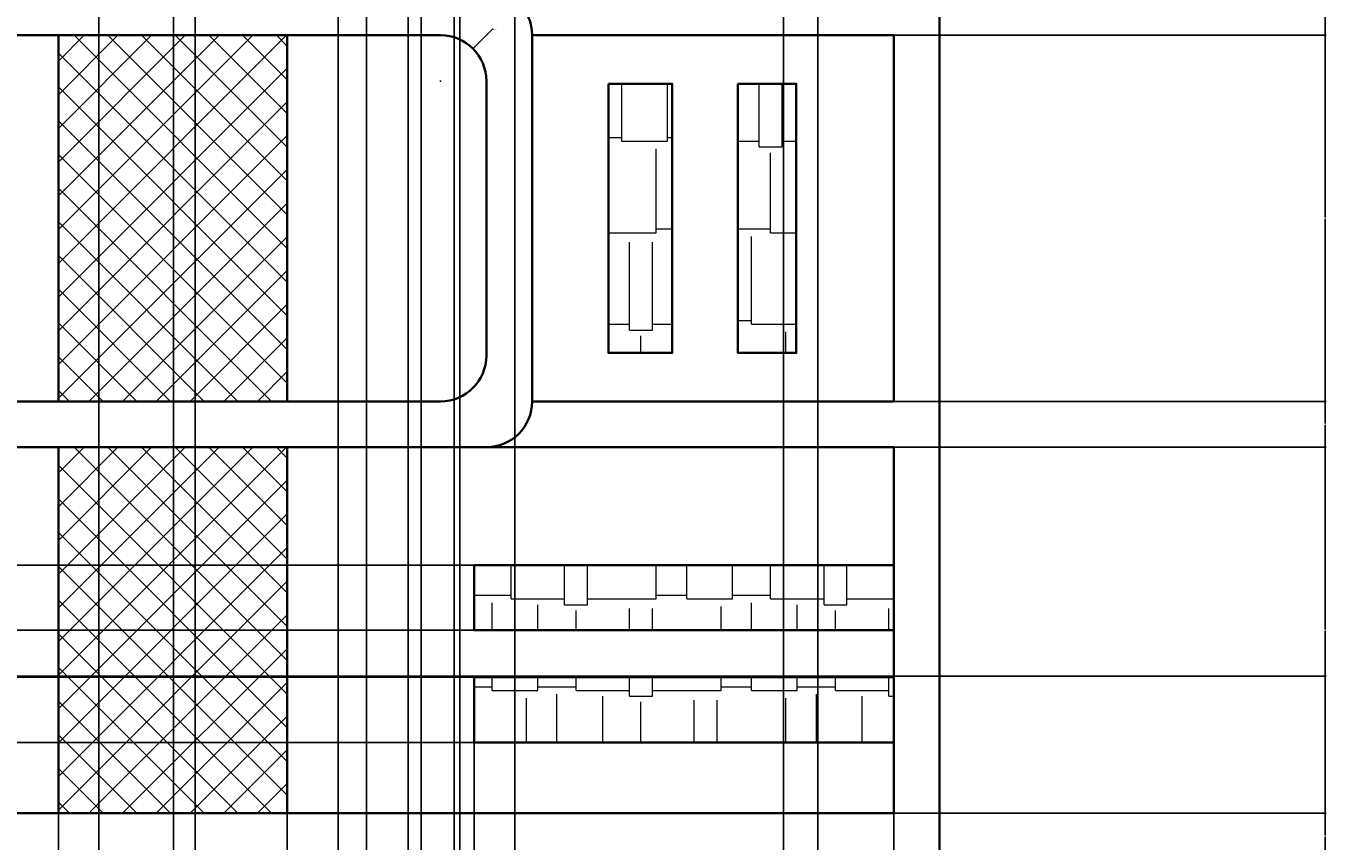
# Model space of a CAD drawing. Units: inches. Extents: x -15 to 605, y -220 to 570.
# Tile 6 of 10: x 265 to 605, y 9 to 222. Entities that reach past the tile are written whole.
import ezdxf

# ---------------------------------------------------------------- set-up
doc = ezdxf.new("R2010")
doc.units = ezdxf.units.IN
doc.header["$MEASUREMENT"] = 0
for name, color, linetype, lineweight in [('A-ANNO-DIMS', 2, 'Continuous', 18), ('A-ELEV', 7, 'Continuous', 35), ('A-ELEV-PATT', 8, 'Continuous', 13)]:
    doc.layers.add(name, color=color, linetype=linetype, lineweight=lineweight)
doc.styles.get("Standard").update_dxf_attribs({"font": 'arial.ttf'})
doc.dimstyles.get("Standard").update_dxf_attribs({"dimtxt": 0.18, "dimasz": 0.18, "dimexe": 0.18, "dimexo": 0.0625, "dimgap": 0.09, "dimtad": 0, "dimtih": 1, "dimtoh": 1, "dimdec": 4, "dimzin": 0, "dimdsep": 46, "dimtxsty": 'Standard', "dimcen": 0.09, "dimadec": 0, "dimazin": 0, "dimtfac": 1, "dimtdec": 4, "dimtofl": 0, "dimtmove": 0, "dimatfit": 3, "dimfxl": 1, "dimtolj": 1, "dimtzin": 0, "dimarcsym": 0})

# ---------------------------------------------------------------- blocks, each defined once
blk = doc.blocks.new('*D8')
at = {"layer": 'A-ANNO-DIMS', "color": 0, "lineweight": -2, "transparency": 16777216}
for p, q in [((23.99, 3.88), (23.99, 570.4)), ((24.17, 570.22), (263.7, 570.22)), ((503.81, 570.22), (264.28, 570.22)), ((503.99, 531.88), (503.99, 570.4))]:
    blk.add_line(p, q, dxfattribs=at)
at = {"layer": 'A-ANNO-DIMS', "color": 0, "transparency": 16777216}
for points in [[(24.17, 570.25), (24.17, 570.19), (23.99, 570.22)], [(503.81, 570.25), (503.81, 570.19), (503.99, 570.22)]]:
    blk.add_solid(points, dxfattribs=at)
at = {"layer": 'Defpoints', "color": 0, "transparency": 16777216}
for p in [(503.99, 570.22), (503.99, 531.82), (23.99, 3.82)]:
    blk.add_point(p, dxfattribs=at)
at = {"layer": 'A-ANNO-DIMS', "color": 0, "transparency": 16777216, "insert": (263.99, 570.22), "char_height": 0.18, "attachment_point": 5}
blk.add_mtext('\\A1;480', dxfattribs=at)
blk = doc.blocks.new('*D9')
at = {"layer": 'A-ANNO-DIMS', "color": 0, "lineweight": -2, "transparency": 16777216}
for p, q in [((503.92, 531.82), (-14.59, 531.82)), ((-14.41, 531.64), (-14.41, 208)), ((-14.41, -116), (-14.41, 207.64)), ((23.92, -116.18), (-14.59, -116.18))]:
    blk.add_line(p, q, dxfattribs=at)
at = {"layer": 'A-ANNO-DIMS', "color": 0, "transparency": 16777216}
for points in [[(-14.44, 531.64), (-14.38, 531.64), (-14.41, 531.82)], [(-14.44, -116), (-14.38, -116), (-14.41, -116.18)]]:
    blk.add_solid(points, dxfattribs=at)
at = {"layer": 'Defpoints', "color": 0, "transparency": 16777216}
for p in [(-14.41, 531.82), (503.99, 531.82), (23.99, -116.18)]:
    blk.add_point(p, dxfattribs=at)
at = {"layer": 'A-ANNO-DIMS', "color": 0, "transparency": 16777216, "insert": (-14.41, 207.82), "char_height": 0.18, "attachment_point": 5}
blk.add_mtext('\\A1;648', dxfattribs=at)
blk = doc.blocks.new('*D11')
at = {"layer": 'A-ANNO-DIMS', "color": 0, "lineweight": -2, "transparency": 16777216}
for p, q in [((492.05, 15.82), (605.3, 15.82)), ((605.12, 15.64), (605.12, 10)), ((605.12, 4), (605.12, 9.64)), ((504.05, 3.82), (605.3, 3.82))]:
    blk.add_line(p, q, dxfattribs=at)
at = {"layer": 'A-ANNO-DIMS', "color": 0, "transparency": 16777216}
for points in [[(605.09, 15.64), (605.15, 15.64), (605.12, 15.82)], [(605.09, 4), (605.15, 4), (605.12, 3.82)]]:
    blk.add_solid(points, dxfattribs=at)
at = {"layer": 'Defpoints', "color": 0, "transparency": 16777216}
for p in [(491.99, 15.82), (605.12, 15.82), (503.99, 3.82)]:
    blk.add_point(p, dxfattribs=at)
at = {"layer": 'A-ANNO-DIMS', "color": 0, "transparency": 16777216, "insert": (605.12, 9.82), "char_height": 0.18, "attachment_point": 5}
blk.add_mtext('\\A1;12', dxfattribs=at)
blk = doc.blocks.new('*D12')
at = {"layer": 'A-ANNO-DIMS', "color": 0, "lineweight": -2, "transparency": 16777216}
for p, q in [((492.05, 111.82), (605.3, 111.82)), ((605.12, 111.64), (605.12, 64)), ((605.12, 16), (605.12, 63.64)), ((492.05, 15.82), (605.3, 15.82))]:
    blk.add_line(p, q, dxfattribs=at)
at = {"layer": 'A-ANNO-DIMS', "color": 0, "transparency": 16777216}
for points in [[(605.09, 111.64), (605.15, 111.64), (605.12, 111.82)], [(605.09, 16), (605.15, 16), (605.12, 15.82)]]:
    blk.add_solid(points, dxfattribs=at)
at = {"layer": 'Defpoints', "color": 0, "transparency": 16777216}
for p in [(491.99, 111.82), (605.12, 111.82), (491.99, 15.82)]:
    blk.add_point(p, dxfattribs=at)
at = {"layer": 'A-ANNO-DIMS', "color": 0, "transparency": 16777216, "insert": (605.12, 63.82), "char_height": 0.18, "attachment_point": 5}
blk.add_mtext('\\A1;96', dxfattribs=at)
blk = doc.blocks.new('*D13')
at = {"layer": 'A-ANNO-DIMS', "color": 0, "lineweight": -2, "transparency": 16777216}
for p, q in [((492.05, 123.82), (605.3, 123.82)), ((605.12, 123.64), (605.12, 118)), ((605.12, 112), (605.12, 117.64)), ((492.05, 111.82), (605.3, 111.82))]:
    blk.add_line(p, q, dxfattribs=at)
at = {"layer": 'A-ANNO-DIMS', "color": 0, "transparency": 16777216}
for points in [[(605.09, 123.64), (605.15, 123.64), (605.12, 123.82)], [(605.09, 112), (605.15, 112), (605.12, 111.82)]]:
    blk.add_solid(points, dxfattribs=at)
at = {"layer": 'Defpoints', "color": 0, "transparency": 16777216}
for p in [(491.99, 123.82), (605.12, 123.82), (491.99, 111.82)]:
    blk.add_point(p, dxfattribs=at)
at = {"layer": 'A-ANNO-DIMS', "color": 0, "transparency": 16777216, "insert": (605.12, 117.82), "char_height": 0.18, "attachment_point": 5}
blk.add_mtext('\\A1;12', dxfattribs=at)
blk = doc.blocks.new('*D14')
at = {"layer": 'A-ANNO-DIMS', "color": 0, "lineweight": -2, "transparency": 16777216}
for p, q in [((492.05, 219.82), (605.3, 219.82)), ((605.12, 219.64), (605.12, 172)), ((605.12, 124), (605.12, 171.64)), ((492.05, 123.82), (605.3, 123.82))]:
    blk.add_line(p, q, dxfattribs=at)
at = {"layer": 'A-ANNO-DIMS', "color": 0, "transparency": 16777216}
for points in [[(605.09, 219.64), (605.15, 219.64), (605.12, 219.82)], [(605.09, 124), (605.15, 124), (605.12, 123.82)]]:
    blk.add_solid(points, dxfattribs=at)
at = {"layer": 'Defpoints', "color": 0, "transparency": 16777216}
for p in [(491.99, 219.82), (605.12, 219.82), (491.99, 123.82)]:
    blk.add_point(p, dxfattribs=at)
at = {"layer": 'A-ANNO-DIMS', "color": 0, "transparency": 16777216, "insert": (605.12, 171.82), "char_height": 0.18, "attachment_point": 5}
blk.add_mtext('\\A1;96', dxfattribs=at)
blk = doc.blocks.new('*D15')
at = {"layer": 'A-ANNO-DIMS', "color": 0, "lineweight": -2, "transparency": 16777216}
for p, q in [((492.05, 231.82), (605.3, 231.82)), ((605.12, 231.64), (605.12, 226)), ((605.12, 220), (605.12, 225.64)), ((492.05, 219.82), (605.3, 219.82))]:
    blk.add_line(p, q, dxfattribs=at)
at = {"layer": 'A-ANNO-DIMS', "color": 0, "transparency": 16777216}
for points in [[(605.09, 231.64), (605.15, 231.64), (605.12, 231.82)], [(605.09, 220), (605.15, 220), (605.12, 219.82)]]:
    blk.add_solid(points, dxfattribs=at)
at = {"layer": 'Defpoints', "color": 0, "transparency": 16777216}
for p in [(491.99, 231.82), (605.12, 231.82), (491.99, 219.82)]:
    blk.add_point(p, dxfattribs=at)
at = {"layer": 'A-ANNO-DIMS', "color": 0, "transparency": 16777216, "insert": (605.12, 225.82), "char_height": 0.18, "attachment_point": 5}
blk.add_mtext('\\A1;12', dxfattribs=at)
blk = doc.blocks.new('*D28')
at = {"layer": 'A-ANNO-DIMS', "color": 0, "lineweight": -2, "transparency": 16777216}
for p, q in [((260.99, 15.76), (260.99, -154.76)), ((272.99, 15.76), (272.99, -154.76)), ((261.17, -154.58), (266.78, -154.58)), ((272.81, -154.58), (267.2, -154.58))]:
    blk.add_line(p, q, dxfattribs=at)
at = {"layer": 'A-ANNO-DIMS', "color": 0, "transparency": 16777216}
for points in [[(261.17, -154.55), (261.17, -154.61), (260.99, -154.58)], [(272.81, -154.55), (272.81, -154.61), (272.99, -154.58)]]:
    blk.add_solid(points, dxfattribs=at)
at = {"layer": 'Defpoints', "color": 0, "transparency": 16777216}
for p in [(260.99, 15.82), (272.99, 15.82), (272.99, -154.58)]:
    blk.add_point(p, dxfattribs=at)
at = {"layer": 'A-ANNO-DIMS', "color": 0, "transparency": 16777216, "insert": (266.99, -154.58), "char_height": 0.18, "attachment_point": 5}
blk.add_mtext('\\A1;12', dxfattribs=at)
blk = doc.blocks.new('*D29')
at = {"layer": 'A-ANNO-DIMS', "color": 0, "lineweight": -2, "transparency": 16777216}
for p, q in [((272.99, 15.76), (272.99, -154.76)), ((332.99, 15.76), (332.99, -154.76)), ((273.17, -154.58), (302.77, -154.58)), ((332.81, -154.58), (303.21, -154.58))]:
    blk.add_line(p, q, dxfattribs=at)
at = {"layer": 'A-ANNO-DIMS', "color": 0, "transparency": 16777216}
for points in [[(273.17, -154.55), (273.17, -154.61), (272.99, -154.58)], [(332.81, -154.55), (332.81, -154.61), (332.99, -154.58)]]:
    blk.add_solid(points, dxfattribs=at)
at = {"layer": 'Defpoints', "color": 0, "transparency": 16777216}
for p in [(272.99, 15.82), (332.99, 15.82), (332.99, -154.58)]:
    blk.add_point(p, dxfattribs=at)
at = {"layer": 'A-ANNO-DIMS', "color": 0, "transparency": 16777216, "insert": (302.99, -154.58), "char_height": 0.18, "attachment_point": 5}
blk.add_mtext('\\A1;60', dxfattribs=at)
blk = doc.blocks.new('*D30')
at = {"layer": 'A-ANNO-DIMS', "color": 0, "lineweight": -2, "transparency": 16777216}
for p, q in [((382.03, 34.31), (382.03, -154.76)), ((332.99, 15.76), (332.99, -154.76)), ((333.17, -154.58), (357.11, -154.58)), ((381.85, -154.58), (357.91, -154.58))]:
    blk.add_line(p, q, dxfattribs=at)
at = {"layer": 'A-ANNO-DIMS', "color": 0, "transparency": 16777216}
for points in [[(333.17, -154.55), (333.17, -154.61), (332.99, -154.58)], [(381.85, -154.55), (381.85, -154.61), (382.03, -154.58)]]:
    blk.add_solid(points, dxfattribs=at)
at = {"layer": 'Defpoints', "color": 0, "transparency": 16777216}
for p in [(382.03, 34.38), (332.99, 15.82), (382.03, -154.58)]:
    blk.add_point(p, dxfattribs=at)
at = {"layer": 'A-ANNO-DIMS', "color": 0, "transparency": 16777216, "insert": (357.51, -154.58), "char_height": 0.18, "attachment_point": 5}
blk.add_mtext('\\A1;49.04', dxfattribs=at)
blk = doc.blocks.new('*D31')
at = {"layer": 'A-ANNO-DIMS', "color": 0, "lineweight": -2, "transparency": 16777216}
for p, q in [((382.03, 34.31), (382.03, -154.76)), ((491.99, 15.76), (491.99, -154.76)), ((382.21, -154.58), (436.55, -154.58)), ((491.81, -154.58), (437.46, -154.58))]:
    blk.add_line(p, q, dxfattribs=at)
at = {"layer": 'A-ANNO-DIMS', "color": 0, "transparency": 16777216}
for points in [[(382.21, -154.55), (382.21, -154.61), (382.03, -154.58)], [(491.81, -154.55), (491.81, -154.61), (491.99, -154.58)]]:
    blk.add_solid(points, dxfattribs=at)
at = {"layer": 'Defpoints', "color": 0, "transparency": 16777216}
for p in [(382.03, 34.38), (491.99, 15.82), (491.99, -154.58)]:
    blk.add_point(p, dxfattribs=at)
at = {"layer": 'A-ANNO-DIMS', "color": 0, "transparency": 16777216, "insert": (437.01, -154.58), "char_height": 0.18, "attachment_point": 5}
blk.add_mtext('\\A1;109.96', dxfattribs=at)
blk = doc.blocks.new('*D32')
at = {"layer": 'A-ANNO-DIMS', "color": 0, "lineweight": -2, "transparency": 16777216}
for p, q in [((491.99, 15.76), (491.99, -154.76)), ((503.99, 3.76), (503.99, -154.76)), ((492.17, -154.58), (497.78, -154.58)), ((503.81, -154.58), (498.2, -154.58))]:
    blk.add_line(p, q, dxfattribs=at)
at = {"layer": 'A-ANNO-DIMS', "color": 0, "transparency": 16777216}
for points in [[(492.17, -154.55), (492.17, -154.61), (491.99, -154.58)], [(503.81, -154.55), (503.81, -154.61), (503.99, -154.58)]]:
    blk.add_solid(points, dxfattribs=at)
at = {"layer": 'Defpoints', "color": 0, "transparency": 16777216}
for p in [(491.99, 15.82), (503.99, 3.82), (503.99, -154.58)]:
    blk.add_point(p, dxfattribs=at)
at = {"layer": 'A-ANNO-DIMS', "color": 0, "transparency": 16777216, "insert": (497.99, -154.58), "char_height": 0.18, "attachment_point": 5}
blk.add_mtext('\\A1;12', dxfattribs=at)
blk = doc.blocks.new('*D33')
at = {"layer": 'A-ANNO-DIMS', "color": 0, "lineweight": -2, "transparency": 16777216}
for p, q in [((491.92, 34.38), (-14.59, 34.38)), ((-14.41, 34.2), (-14.41, 25.28)), ((-14.41, 16), (-14.41, 24.92)), ((491.92, 15.82), (-14.59, 15.82))]:
    blk.add_line(p, q, dxfattribs=at)
at = {"layer": 'A-ANNO-DIMS', "color": 0, "transparency": 16777216}
for points in [[(-14.44, 34.2), (-14.38, 34.2), (-14.41, 34.38)], [(-14.44, 16), (-14.38, 16), (-14.41, 15.82)]]:
    blk.add_solid(points, dxfattribs=at)
at = {"layer": 'Defpoints', "color": 0, "transparency": 16777216}
for p in [(-14.41, 34.38), (491.99, 34.38), (491.99, 15.82)]:
    blk.add_point(p, dxfattribs=at)
at = {"layer": 'A-ANNO-DIMS', "color": 0, "transparency": 16777216, "insert": (-14.41, 25.1), "char_height": 0.18, "attachment_point": 5}
blk.add_mtext('\\A1;18.557', dxfattribs=at)
blk = doc.blocks.new('*D34')
at = {"layer": 'A-ANNO-DIMS', "color": 0, "lineweight": -2, "transparency": 16777216}
for p, q in [((491.92, 51.48), (-14.59, 51.48)), ((-14.41, 51.3), (-14.41, 43.11)), ((-14.41, 34.56), (-14.41, 42.75)), ((491.92, 34.38), (-14.59, 34.38))]:
    blk.add_line(p, q, dxfattribs=at)
at = {"layer": 'A-ANNO-DIMS', "color": 0, "transparency": 16777216}
for points in [[(-14.44, 51.3), (-14.38, 51.3), (-14.41, 51.48)], [(-14.44, 34.56), (-14.38, 34.56), (-14.41, 34.38)]]:
    blk.add_solid(points, dxfattribs=at)
at = {"layer": 'Defpoints', "color": 0, "transparency": 16777216}
for p in [(-14.41, 51.48), (491.99, 51.48), (491.99, 34.38)]:
    blk.add_point(p, dxfattribs=at)
at = {"layer": 'A-ANNO-DIMS', "color": 0, "transparency": 16777216, "insert": (-14.41, 42.93), "char_height": 0.18, "attachment_point": 5}
blk.add_mtext('\\A1;17.1', dxfattribs=at)
blk = doc.blocks.new('*D35')
at = {"layer": 'A-ANNO-DIMS', "color": 0, "lineweight": -2, "transparency": 16777216}
for p, q in [((491.92, 63.82), (-14.59, 63.82)), ((-14.41, 63.64), (-14.41, 57.83)), ((-14.41, 51.66), (-14.41, 57.47)), ((491.92, 51.48), (-14.59, 51.48))]:
    blk.add_line(p, q, dxfattribs=at)
at = {"layer": 'A-ANNO-DIMS', "color": 0, "transparency": 16777216}
for points in [[(-14.44, 63.64), (-14.38, 63.64), (-14.41, 63.82)], [(-14.44, 51.66), (-14.38, 51.66), (-14.41, 51.48)]]:
    blk.add_solid(points, dxfattribs=at)
at = {"layer": 'Defpoints', "color": 0, "transparency": 16777216}
for p in [(-14.41, 63.82), (491.99, 63.82), (491.99, 51.48)]:
    blk.add_point(p, dxfattribs=at)
at = {"layer": 'A-ANNO-DIMS', "color": 0, "transparency": 16777216, "insert": (-14.41, 57.65), "char_height": 0.18, "attachment_point": 5}
blk.add_mtext('\\A1;12.342', dxfattribs=at)
blk = doc.blocks.new('*D36')
at = {"layer": 'A-ANNO-DIMS', "color": 0, "lineweight": -2, "transparency": 16777216}
for p, q in [((491.92, 80.92), (-14.59, 80.92)), ((-14.41, 80.74), (-14.41, 72.55)), ((-14.41, 64), (-14.41, 72.19)), ((491.92, 63.82), (-14.59, 63.82))]:
    blk.add_line(p, q, dxfattribs=at)
at = {"layer": 'A-ANNO-DIMS', "color": 0, "transparency": 16777216}
for points in [[(-14.44, 80.74), (-14.38, 80.74), (-14.41, 80.92)], [(-14.44, 64), (-14.38, 64), (-14.41, 63.82)]]:
    blk.add_solid(points, dxfattribs=at)
at = {"layer": 'Defpoints', "color": 0, "transparency": 16777216}
for p in [(-14.41, 80.92), (491.99, 80.92), (491.99, 63.82)]:
    blk.add_point(p, dxfattribs=at)
at = {"layer": 'A-ANNO-DIMS', "color": 0, "transparency": 16777216, "insert": (-14.41, 72.37), "char_height": 0.18, "attachment_point": 5}
blk.add_mtext('\\A1;17.1', dxfattribs=at)
blk = doc.blocks.new('*D37')
at = {"layer": 'A-ANNO-DIMS', "color": 0, "lineweight": -2, "transparency": 16777216}
for p, q in [((129.05, 51.82), (605.3, 51.82)), ((605.12, 51.64), (605.12, 34)), ((605.12, 16), (605.12, 33.64)), ((129.05, 15.82), (605.3, 15.82))]:
    blk.add_line(p, q, dxfattribs=at)
at = {"layer": 'A-ANNO-DIMS', "color": 0, "transparency": 16777216}
for points in [[(605.09, 51.64), (605.15, 51.64), (605.12, 51.82)], [(605.09, 16), (605.15, 16), (605.12, 15.82)]]:
    blk.add_solid(points, dxfattribs=at)
at = {"layer": 'Defpoints', "color": 0, "transparency": 16777216}
for p in [(128.99, 51.82), (605.12, 51.82), (128.99, 15.82)]:
    blk.add_point(p, dxfattribs=at)
at = {"layer": 'A-ANNO-DIMS', "color": 0, "transparency": 16777216, "insert": (605.12, 33.82), "char_height": 0.18, "attachment_point": 5}
blk.add_mtext('\\A1;36', dxfattribs=at)
blk = doc.blocks.new('*D56')
at = {"layer": 'A-ANNO-DIMS', "color": 0, "lineweight": -2, "transparency": 16777216}
for p, q in [((233.14, -31.58), (233.14, 570.4)), ((233.32, 570.22), (298.47, 570.22)), ((364.53, 570.22), (299.38, 570.22)), ((364.71, -56.12), (364.71, 570.4))]:
    blk.add_line(p, q, dxfattribs=at)
at = {"layer": 'A-ANNO-DIMS', "color": 0, "transparency": 16777216}
for points in [[(233.32, 570.25), (233.32, 570.19), (233.14, 570.22)], [(364.53, 570.25), (364.53, 570.19), (364.71, 570.22)]]:
    blk.add_solid(points, dxfattribs=at)
at = {"layer": 'Defpoints', "color": 0, "transparency": 16777216}
for p in [(364.71, 570.22), (233.14, -31.64), (364.71, -56.18)]:
    blk.add_point(p, dxfattribs=at)
at = {"layer": 'A-ANNO-DIMS', "color": 0, "transparency": 16777216, "insert": (298.93, 570.22), "char_height": 0.18, "attachment_point": 5}
blk.add_mtext('\\A1;131.56', dxfattribs=at)
blk = doc.blocks.new('*D57')
at = {"layer": 'A-ANNO-DIMS', "color": 0, "lineweight": -2, "transparency": 16777216}
for p, q in [((364.71, -56.12), (364.71, 570.4)), ((364.89, 570.22), (370.5, 570.22)), ((376.53, 570.22), (370.92, 570.22)), ((376.71, -44.82), (376.71, 570.4))]:
    blk.add_line(p, q, dxfattribs=at)
at = {"layer": 'A-ANNO-DIMS', "color": 0, "transparency": 16777216}
for points in [[(364.89, 570.25), (364.89, 570.19), (364.71, 570.22)], [(376.53, 570.25), (376.53, 570.19), (376.71, 570.22)]]:
    blk.add_solid(points, dxfattribs=at)
at = {"layer": 'Defpoints', "color": 0, "transparency": 16777216}
for p in [(376.71, 570.22), (376.71, -44.88), (364.71, -56.18)]:
    blk.add_point(p, dxfattribs=at)
at = {"layer": 'A-ANNO-DIMS', "color": 0, "transparency": 16777216, "insert": (370.71, 570.22), "char_height": 0.18, "attachment_point": 5}
blk.add_mtext('\\A1;12', dxfattribs=at)
blk = doc.blocks.new('*D58')
at = {"layer": 'A-ANNO-DIMS', "color": 0, "lineweight": -2, "transparency": 16777216}
for p, q in [((376.71, -44.82), (376.71, 570.4)), ((376.89, 570.22), (419.58, 570.22)), ((462.92, 570.22), (420.23, 570.22)), ((463.1, -45.87), (463.1, 570.4))]:
    blk.add_line(p, q, dxfattribs=at)
at = {"layer": 'A-ANNO-DIMS', "color": 0, "transparency": 16777216}
for points in [[(376.89, 570.25), (376.89, 570.19), (376.71, 570.22)], [(462.92, 570.25), (462.92, 570.19), (463.1, 570.22)]]:
    blk.add_solid(points, dxfattribs=at)
at = {"layer": 'Defpoints', "color": 0, "transparency": 16777216}
for p in [(463.1, 570.22), (376.71, -44.88), (463.1, -45.94)]:
    blk.add_point(p, dxfattribs=at)
at = {"layer": 'A-ANNO-DIMS', "color": 0, "transparency": 16777216, "insert": (419.9, 570.22), "char_height": 0.18, "attachment_point": 5}
blk.add_mtext('\\A1;86.4', dxfattribs=at)
blk = doc.blocks.new('*D59')
at = {"layer": 'A-ANNO-DIMS', "color": 0, "lineweight": -2, "transparency": 16777216}
for p, q in [((463.1, -45.87), (463.1, 570.4)), ((463.28, 570.22), (467.45, 570.22)), ((471.92, 570.22), (467.75, 570.22)), ((472.1, -45.87), (472.1, 570.4))]:
    blk.add_line(p, q, dxfattribs=at)
at = {"layer": 'A-ANNO-DIMS', "color": 0, "transparency": 16777216}
for points in [[(463.28, 570.25), (463.28, 570.19), (463.1, 570.22)], [(471.92, 570.25), (471.92, 570.19), (472.1, 570.22)]]:
    blk.add_solid(points, dxfattribs=at)
at = {"layer": 'Defpoints', "color": 0, "transparency": 16777216}
for p in [(472.1, 570.22), (463.1, -45.94), (472.1, -45.94)]:
    blk.add_point(p, dxfattribs=at)
at = {"layer": 'A-ANNO-DIMS', "color": 0, "transparency": 16777216, "insert": (467.6, 570.22), "char_height": 0.18, "attachment_point": 5}
blk.add_mtext('\\A1;9', dxfattribs=at)
blk = doc.blocks.new('*D60')
at = {"layer": 'A-ANNO-DIMS', "color": 0, "lineweight": -2, "transparency": 16777216}
for p, q in [((346.37, -116.12), (346.37, 570.4)), ((346.55, 570.22), (349.67, 570.22)), ((353.57, 570.22), (350.45, 570.22)), ((353.75, -39.82), (353.75, 570.4))]:
    blk.add_line(p, q, dxfattribs=at)
at = {"layer": 'A-ANNO-DIMS', "color": 0, "transparency": 16777216}
for points in [[(346.55, 570.25), (346.55, 570.19), (346.37, 570.22)], [(353.57, 570.25), (353.57, 570.19), (353.75, 570.22)]]:
    blk.add_solid(points, dxfattribs=at)
at = {"layer": 'Defpoints', "color": 0, "transparency": 16777216}
for p in [(353.75, 570.22), (353.75, -39.88), (346.37, -116.18)]:
    blk.add_point(p, dxfattribs=at)
at = {"layer": 'A-ANNO-DIMS', "color": 0, "transparency": 16777216, "insert": (350.06, 570.22), "char_height": 0.18, "attachment_point": 5}
blk.add_mtext('\\A1;7.384', dxfattribs=at)
blk = doc.blocks.new('*D61')
at = {"layer": 'A-ANNO-DIMS', "color": 0, "lineweight": -2, "transparency": 16777216}
for p, q in [((353.75, -39.82), (353.75, 570.4)), ((353.93, 570.22), (360.55, 570.22)), ((367.95, 570.22), (361.33, 570.22)), ((368.13, -39.82), (368.13, 570.4))]:
    blk.add_line(p, q, dxfattribs=at)
at = {"layer": 'A-ANNO-DIMS', "color": 0, "transparency": 16777216}
for points in [[(353.93, 570.25), (353.93, 570.19), (353.75, 570.22)], [(367.95, 570.25), (367.95, 570.19), (368.13, 570.22)]]:
    blk.add_solid(points, dxfattribs=at)
at = {"layer": 'Defpoints', "color": 0, "transparency": 16777216}
for p in [(368.13, 570.22), (353.75, -39.88), (368.13, -39.88)]:
    blk.add_point(p, dxfattribs=at)
at = {"layer": 'A-ANNO-DIMS', "color": 0, "transparency": 16777216, "insert": (360.94, 570.22), "char_height": 0.18, "attachment_point": 5}
blk.add_mtext('\\A1;14.38', dxfattribs=at)
blk = doc.blocks.new('*D62')
at = {"layer": 'A-ANNO-DIMS', "color": 0, "lineweight": -2, "transparency": 16777216}
for p, q in [((378.23, -39.82), (378.23, 570.4)), ((378.41, 570.22), (385.04, 570.22)), ((392.43, 570.22), (385.81, 570.22)), ((392.61, -39.82), (392.61, 570.4))]:
    blk.add_line(p, q, dxfattribs=at)
at = {"layer": 'A-ANNO-DIMS', "color": 0, "transparency": 16777216}
for points in [[(378.41, 570.25), (378.41, 570.19), (378.23, 570.22)], [(392.43, 570.25), (392.43, 570.19), (392.61, 570.22)]]:
    blk.add_solid(points, dxfattribs=at)
at = {"layer": 'Defpoints', "color": 0, "transparency": 16777216}
for p in [(392.61, 570.22), (378.23, -39.88), (392.61, -39.88)]:
    blk.add_point(p, dxfattribs=at)
at = {"layer": 'A-ANNO-DIMS', "color": 0, "transparency": 16777216, "insert": (385.42, 570.22), "char_height": 0.18, "attachment_point": 5}
blk.add_mtext('\\A1;14.38', dxfattribs=at)
blk = doc.blocks.new('*D98')
at = {"layer": 'A-ANNO-DIMS', "color": 0, "lineweight": -2, "transparency": 16777216}
for p, q in [((386.77, 221.4), (381.8, 216.43)), ((386.95, 221.4), (386.77, 221.4)), ((373.19, 207.73), (373.19, 207.91)), ((373.1, 207.82), (373.28, 207.82))]:
    blk.add_line(p, q, dxfattribs=at)
at = {"layer": 'A-ANNO-DIMS', "color": 0, "transparency": 16777216}
blk.add_solid([(381.78, 216.45), (381.83, 216.41), (381.68, 216.3)], dxfattribs=at)
at = {"layer": 'Defpoints', "color": 0, "transparency": 16777216}
for p in [(381.68, 216.3), (373.19, 207.82)]:
    blk.add_point(p, dxfattribs=at)
at = {"layer": 'A-ANNO-DIMS', "color": 0, "transparency": 16777216, "insert": (387.45, 221.4), "char_height": 0.18, "attachment_point": 5}
blk.add_mtext('\\A1;8X R12', dxfattribs=at)
blk = doc.blocks.new('*D104')
at = {"layer": 'A-ANNO-DIMS', "color": 0, "lineweight": -2, "transparency": 16777216}
for p, q in [((251.99, -56.12), (251.99, 570.4)), ((252.17, 570.22), (267.39, 570.22)), ((283.41, 570.22), (268.18, 570.22)), ((283.59, -84.79), (283.59, 570.4))]:
    blk.add_line(p, q, dxfattribs=at)
at = {"layer": 'A-ANNO-DIMS', "color": 0, "transparency": 16777216}
for points in [[(252.17, 570.25), (252.17, 570.19), (251.99, 570.22)], [(283.41, 570.25), (283.41, 570.19), (283.59, 570.22)]]:
    blk.add_solid(points, dxfattribs=at)
at = {"layer": 'Defpoints', "color": 0, "transparency": 16777216}
for p in [(283.59, 570.22), (251.99, -56.18), (283.59, -84.86)]:
    blk.add_point(p, dxfattribs=at)
at = {"layer": 'A-ANNO-DIMS', "color": 0, "transparency": 16777216, "insert": (267.79, 570.22), "char_height": 0.18, "attachment_point": 5}
blk.add_mtext('\\A1;31.60', dxfattribs=at)
blk = doc.blocks.new('*D105')
at = {"layer": 'A-ANNO-DIMS', "color": 0, "lineweight": -2, "transparency": 16777216}
for p, q in [((283.59, -84.79), (283.59, 570.4)), ((283.77, 570.22), (292.92, 570.22)), ((302.99, 570.22), (293.84, 570.22)), ((303.17, -103.62), (303.17, 570.4))]:
    blk.add_line(p, q, dxfattribs=at)
at = {"layer": 'A-ANNO-DIMS', "color": 0, "transparency": 16777216}
for points in [[(283.77, 570.25), (283.77, 570.19), (283.59, 570.22)], [(302.99, 570.25), (302.99, 570.19), (303.17, 570.22)]]:
    blk.add_solid(points, dxfattribs=at)
at = {"layer": 'Defpoints', "color": 0, "transparency": 16777216}
for p in [(303.17, 570.22), (283.59, -84.86), (303.17, -103.68)]:
    blk.add_point(p, dxfattribs=at)
at = {"layer": 'A-ANNO-DIMS', "color": 0, "transparency": 16777216, "insert": (293.38, 570.22), "char_height": 0.18, "attachment_point": 5}
blk.add_mtext('\\A1;19.585', dxfattribs=at)
blk = doc.blocks.new('*D106')
at = {"layer": 'A-ANNO-DIMS', "color": 0, "lineweight": -2, "transparency": 16777216}
for p, q in [((303.17, -103.62), (303.17, 570.4)), ((303.35, 570.22), (305.62, 570.22)), ((308.68, 570.22), (306.41, 570.22)), ((308.86, -79.16), (308.86, 570.4))]:
    blk.add_line(p, q, dxfattribs=at)
at = {"layer": 'A-ANNO-DIMS', "color": 0, "transparency": 16777216}
for points in [[(303.35, 570.25), (303.35, 570.19), (303.17, 570.22)], [(308.68, 570.25), (308.68, 570.19), (308.86, 570.22)]]:
    blk.add_solid(points, dxfattribs=at)
at = {"layer": 'Defpoints', "color": 0, "transparency": 16777216}
for p in [(308.86, 570.22), (308.86, -79.22), (303.17, -103.68)]:
    blk.add_point(p, dxfattribs=at)
at = {"layer": 'A-ANNO-DIMS', "color": 0, "transparency": 16777216, "insert": (306.02, 570.22), "char_height": 0.18, "attachment_point": 5}
blk.add_mtext('\\A1;5.689', dxfattribs=at)

msp = doc.modelspace()

# ---------------------------------------------------------------- hatches: boundary and pattern name
at = {"layer": 'A-ELEV-PATT'}
h = msp.add_hatch(dxfattribs=at)
h.set_pattern_fill('AR-RSHKE', color=256, scale=2)
h.set_pattern_definition([(0, (-191.319, 0), (51, 24), [12, -10, 14, -6, 18, -8]), (0, (-179.319, 1), (51, 24), [10, -38, 8, -12]), (0, (-155.319, -1.5), (51, 24), [6, -62]), (90, (-191.319, 0), (-17, 24), [23, -73]), (90, (-179.319, 0), (-17, 24), [22.5, -73.5]), (90, (-169.319, 0), (-17, 24), [21, -75]), (90, (-155.319, -1.5), (-17, 24), [23, -73]), (90, (-149.319, -1.5), (-17, 24), [23, -73]), (90, (-131.319, 0), (-17, 24), [22, -74])])
h.paths.add_polyline_path([(491.9872, 80.9192), (382.0304, 80.9192), (382.0304, 63.8187), (491.9872, 63.8187)])
h.paths.add_polyline_path([(491.9872, 51.4763), (382.0304, 51.4763), (382.0304, 34.3758), (491.9872, 34.3758)])
h.paths.add_polyline_path([(433.9097, 207.1093), (417.1672, 207.1093), (417.1672, 136.5115), (433.9097, 136.5115)])
h.paths.add_polyline_path([(466.4098, 207.1093), (451.1446, 207.1093), (451.1446, 136.5115), (466.4098, 136.5115)])
h.paths.add_polyline_path([(491.9872, 296.9192), (382.0304, 296.9192), (382.0304, 279.8187), (491.9872, 279.8187)])
h.paths.add_polyline_path([(491.9872, 267.4763), (382.0304, 267.4763), (382.0304, 250.3758), (491.9872, 250.3758)])
h.paths.add_polyline_path([(433.9097, 423.1093), (417.1672, 423.1093), (417.1672, 352.5115), (433.9097, 352.5115)])
h.paths.add_polyline_path([(466.4098, 423.1093), (451.1446, 423.1093), (451.1446, 352.5115), (466.4098, 352.5115)])
h = msp.add_hatch(dxfattribs=at)
h.set_pattern_fill('ANSI37', color=256, scale=50)
h.set_pattern_definition([(45, (0, 108), (-4.41942, 4.41942), []), (135, (0, 108), (-4.41942, -4.41942), [])])
h.paths.add_polyline_path([(332.9872, 219.8187), (272.9872, 219.8187), (272.9872, 123.8187), (332.9872, 123.8187)])
h = msp.add_hatch(dxfattribs=at)
h.set_pattern_fill('ANSI37', color=256, scale=50)
h.paths.add_polyline_path([(332.9872, 111.8187), (272.9872, 111.8187), (272.9872, 15.8187), (332.9872, 15.8187)])

# ---------------------------------------------------------------- linework, layer by layer
at = {"layer": 'A-ELEV'}
for p, q in [((373.1921, 219.8187), (44.9872, 219.8187)), ((272.9872, 219.8187), (272.9872, 123.8187)), ((332.9872, 219.8187), (332.9872, 123.8187)), ((397.1921, 123.8187), (397.1921, 219.8187)), ((397.1921, 219.8187), (491.9872, 219.8187)), ((491.9872, 123.8187), (491.9872, 219.8187)), ((385.1921, 135.8187), (385.1921, 207.8187)), ((373.1921, 123.8187), (44.9872, 123.8187)), ((260.9872, 123.8187), (373.1921, 123.8187)), ((491.9872, 123.8187), (397.1921, 123.8187)), ((491.9872, 111.8187), (140.9872, 111.8187)), ((272.9872, 111.8187), (272.9872, 15.8187)), ((332.9872, 111.8187), (332.9872, 15.8187)), ((491.9872, 15.8187), (491.9872, 111.8187)), ((260.9872, 15.8187), (491.9872, 15.8187))]:
    msp.add_line(p, q, dxfattribs=at)
msp.add_lwpolyline([(23.9872, 123.8187), (23.9872, 3.8187), (503.9872, 3.8187), (503.9872, 123.8187), (503.9872, 531.8187)], dxfattribs=at)
for points in [[(417.1672, 207.1093), (433.9097, 207.1093), (433.9097, 136.5115), (417.1672, 136.5115)], [(451.1446, 207.1093), (466.4098, 207.1093), (466.4098, 136.5115), (451.1446, 136.5115)], [(491.9872, 63.8187), (382.0304, 63.8187), (382.0304, 80.9192), (491.9872, 80.9192)], [(491.9872, 34.3758), (382.0304, 34.3758), (382.0304, 51.4763), (491.9872, 51.4763)]]:
    msp.add_lwpolyline(points, close=True, dxfattribs=at)
for centre, start, end in [((385.1921, 219.8187), 0, 90), ((373.1921, 207.8187), 0, 90), ((373.1921, 135.8187), 270, 0), ((385.1921, 123.8187), 270, 0)]:
    msp.add_arc(centre, 12, start, end, dxfattribs=at)

# ---------------------------------------------------------------- dimensions: what is measured, and where the dimension line sits
at = {"layer": 'A-ANNO-DIMS'}
for base, p1, p2, override, picture, middle in [((503.9872, 570.2187), (23.9872, 3.8187), (503.9872, 531.8187), {"dimdec": 0, "dimlfac": 1, "dimrnd": 0, "dimzin": 0, "dimdsep": 46, "dimlunit": 2}, '*D8', (263.9872, 570.2187)), ((364.7066, 570.2187), (233.1439, -31.6396), (364.7066, -56.1813), {"dimdec": 2, "dimlfac": 1, "dimrnd": 0, "dimzin": 0, "dimdsep": 46, "dimlunit": 2}, '*D56', (298.9252, 570.2187)), ((283.5871, 570.2187), (251.9872, -56.1813), (283.5871, -84.8572), {"dimdec": 2, "dimlfac": 1, "dimrnd": 0, "dimzin": 0, "dimdsep": 46, "dimlunit": 2}, '*D104', (267.7872, 570.2187)), ((303.1719, 570.2187), (283.5871, -84.8572), (303.1719, -103.6786), {"dimdec": 3, "dimlfac": 1, "dimrnd": 0, "dimzin": 0, "dimdsep": 46, "dimlunit": 2}, '*D105', (293.3795, 570.2187)), ((308.8611, 570.2187), (303.1719, -103.6786), (308.8611, -79.2202), {"dimdec": 3, "dimlfac": 1, "dimrnd": 0, "dimzin": 0, "dimdsep": 46, "dimlunit": 2}, '*D106', (306.0165, 570.2187)), ((353.7501, 570.2187), (346.3663, -116.1813), (353.7501, -39.8843), {"dimdec": 3, "dimlfac": 1, "dimrnd": 0, "dimzin": 0, "dimdsep": 46, "dimlunit": 2}, '*D60', (350.0582, 570.2187)), ((368.1292, 570.2187), (353.7501, -39.8843), (368.1292, -39.8843), {"dimdec": 2, "dimlfac": 1, "dimrnd": 0, "dimzin": 0, "dimdsep": 46, "dimlunit": 2}, '*D61', (360.9397, 570.2187)), ((376.7066, 570.2187), (364.7066, -56.1813), (376.7066, -44.8803), {"dimdec": 0, "dimlfac": 1, "dimrnd": 0, "dimzin": 0, "dimdsep": 46, "dimlunit": 2}, '*D57', (370.7066, 570.2187)), ((463.1032, 570.2187), (376.7066, -44.8803), (463.1032, -45.9373), {"dimdec": 1, "dimlfac": 1, "dimrnd": 0, "dimzin": 0, "dimdsep": 46, "dimlunit": 2}, '*D58', (419.9049, 570.2187)), ((392.6125, 570.2187), (378.2334, -39.8843), (392.6125, -39.8843), {"dimdec": 2, "dimlfac": 1, "dimrnd": 0, "dimzin": 0, "dimdsep": 46, "dimlunit": 2}, '*D62', (385.423, 570.2187)), ((472.1032, 570.2187), (463.1032, -45.9373), (472.1032, -45.9373), {"dimdec": 0, "dimlfac": 1, "dimrnd": 0, "dimzin": 0, "dimdsep": 46, "dimlunit": 2}, '*D59', (467.6032, 570.2187)), ((382.0304, -154.5813), (332.9872, 15.8187), (382.0304, 34.3758), {"dimdec": 2, "dimlfac": 1, "dimrnd": 0, "dimzin": 0, "dimdsep": 46, "dimlunit": 2}, '*D30', (357.5088, -154.5813)), ((491.9872, -154.5813), (382.0304, 34.3758), (491.9872, 15.8187), {"dimdec": 2, "dimlfac": 1, "dimrnd": 0, "dimzin": 0, "dimdsep": 46, "dimlunit": 2}, '*D31', (437.0088, -154.5813)), ((272.9872, -154.5813), (260.9872, 15.8187), (272.9872, 15.8187), {"dimdec": 0, "dimlfac": 1, "dimrnd": 0, "dimzin": 0, "dimdsep": 46, "dimlunit": 2}, '*D28', (266.9872, -154.5813)), ((332.9872, -154.5813), (272.9872, 15.8187), (332.9872, 15.8187), {"dimdec": 0, "dimlfac": 1, "dimrnd": 0, "dimzin": 0, "dimdsep": 46, "dimlunit": 2}, '*D29', (302.9872, -154.5813)), ((503.9872, -154.5813), (491.9872, 15.8187), (503.9872, 3.8187), {"dimdec": 0, "dimlfac": 1, "dimrnd": 0, "dimzin": 0, "dimdsep": 46, "dimlunit": 2}, '*D32', (497.9872, -154.5813))]:
    dim = msp.add_linear_dim(base=base, p1=p1, p2=p2, dimstyle='Standard', override=override, dxfattribs=at)
    dim.commit()
    dim.dimension.update_dxf_attribs({"geometry": picture, "text_midpoint": middle})
for base, p1, p2, override, picture, middle in [((-14.4128, 531.8187), (23.9872, -116.1813), (503.9872, 531.8187), {"dimdec": 0, "dimlfac": 1, "dimrnd": 0, "dimzin": 0, "dimdsep": 46, "dimlunit": 2}, '*D9', (-14.4128, 207.8187)), ((605.1161, 231.8187), (491.9872, 219.8187), (491.9872, 231.8187), {"dimdec": 0, "dimlfac": 1, "dimrnd": 0, "dimzin": 0, "dimdsep": 46, "dimlunit": 2}, '*D15', (605.1161, 225.8187)), ((605.1161, 219.8187), (491.9872, 123.8187), (491.9872, 219.8187), {"dimdec": 0, "dimlfac": 1, "dimrnd": 0, "dimzin": 0, "dimdsep": 46, "dimlunit": 2}, '*D14', (605.1161, 171.8187)), ((605.1161, 123.8187), (491.9872, 111.8187), (491.9872, 123.8187), {"dimdec": 0, "dimlfac": 1, "dimrnd": 0, "dimzin": 0, "dimdsep": 46, "dimlunit": 2}, '*D13', (605.1161, 117.8187)), ((605.1161, 111.8187), (491.9872, 15.8187), (491.9872, 111.8187), {"dimdec": 0, "dimlfac": 1, "dimrnd": 0, "dimzin": 0, "dimdsep": 46, "dimlunit": 2}, '*D12', (605.1161, 63.8187)), ((-14.4128, 80.9192), (491.9872, 63.8187), (491.9872, 80.9192), {"dimdec": 1, "dimlfac": 1, "dimrnd": 0, "dimzin": 0, "dimdsep": 46, "dimlunit": 2}, '*D36', (-14.4128, 72.369)), ((-14.4128, 63.8187), (491.9872, 51.4763), (491.9872, 63.8187), {"dimdec": 3, "dimlfac": 1, "dimrnd": 0, "dimzin": 0, "dimdsep": 46, "dimlunit": 2}, '*D35', (-14.4128, 57.6475)), ((-14.4128, 51.4763), (491.9872, 34.3758), (491.9872, 51.4763), {"dimdec": 1, "dimlfac": 1, "dimrnd": 0, "dimzin": 0, "dimdsep": 46, "dimlunit": 2}, '*D34', (-14.4128, 42.926)), ((605.1161, 51.8187), (128.9872, 15.8187), (128.9872, 51.8187), {"dimdec": 0, "dimlfac": 1, "dimrnd": 0, "dimzin": 0, "dimdsep": 46, "dimlunit": 2}, '*D37', (605.1161, 33.8187)), ((-14.4128, 34.3758), (491.9872, 15.8187), (491.9872, 34.3758), {"dimdec": 3, "dimlfac": 1, "dimrnd": 0, "dimzin": 0, "dimdsep": 46, "dimlunit": 2}, '*D33', (-14.4128, 25.0973)), ((605.1161, 15.8187), (503.9872, 3.8187), (491.9872, 15.8187), {"dimdec": 0, "dimlfac": 1, "dimrnd": 0, "dimzin": 0, "dimdsep": 46, "dimlunit": 2}, '*D11', (605.1161, 9.8187))]:
    dim = msp.add_linear_dim(base=base, p1=p1, p2=p2, angle=90, dimstyle='Standard', override=override, dxfattribs=at)
    dim.commit()
    dim.dimension.update_dxf_attribs({"geometry": picture, "text_midpoint": middle})
dim = msp.add_radius_dim(center=(373.1921, 207.8187), mpoint=(381.6772, 216.3042), text='8X <>', dimstyle='Standard', override={"dimdec": 0, "dimlfac": 1, "dimrnd": 0, "dimzin": 0, "dimdsep": 46, "dimlunit": 2}, dxfattribs=at)
dim.commit()
dim.dimension.update_dxf_attribs({"geometry": '*D98', "text_midpoint": (387.4459, 221.3955), "dimtype": 164})

doc.saveas('drawing.dxf')
